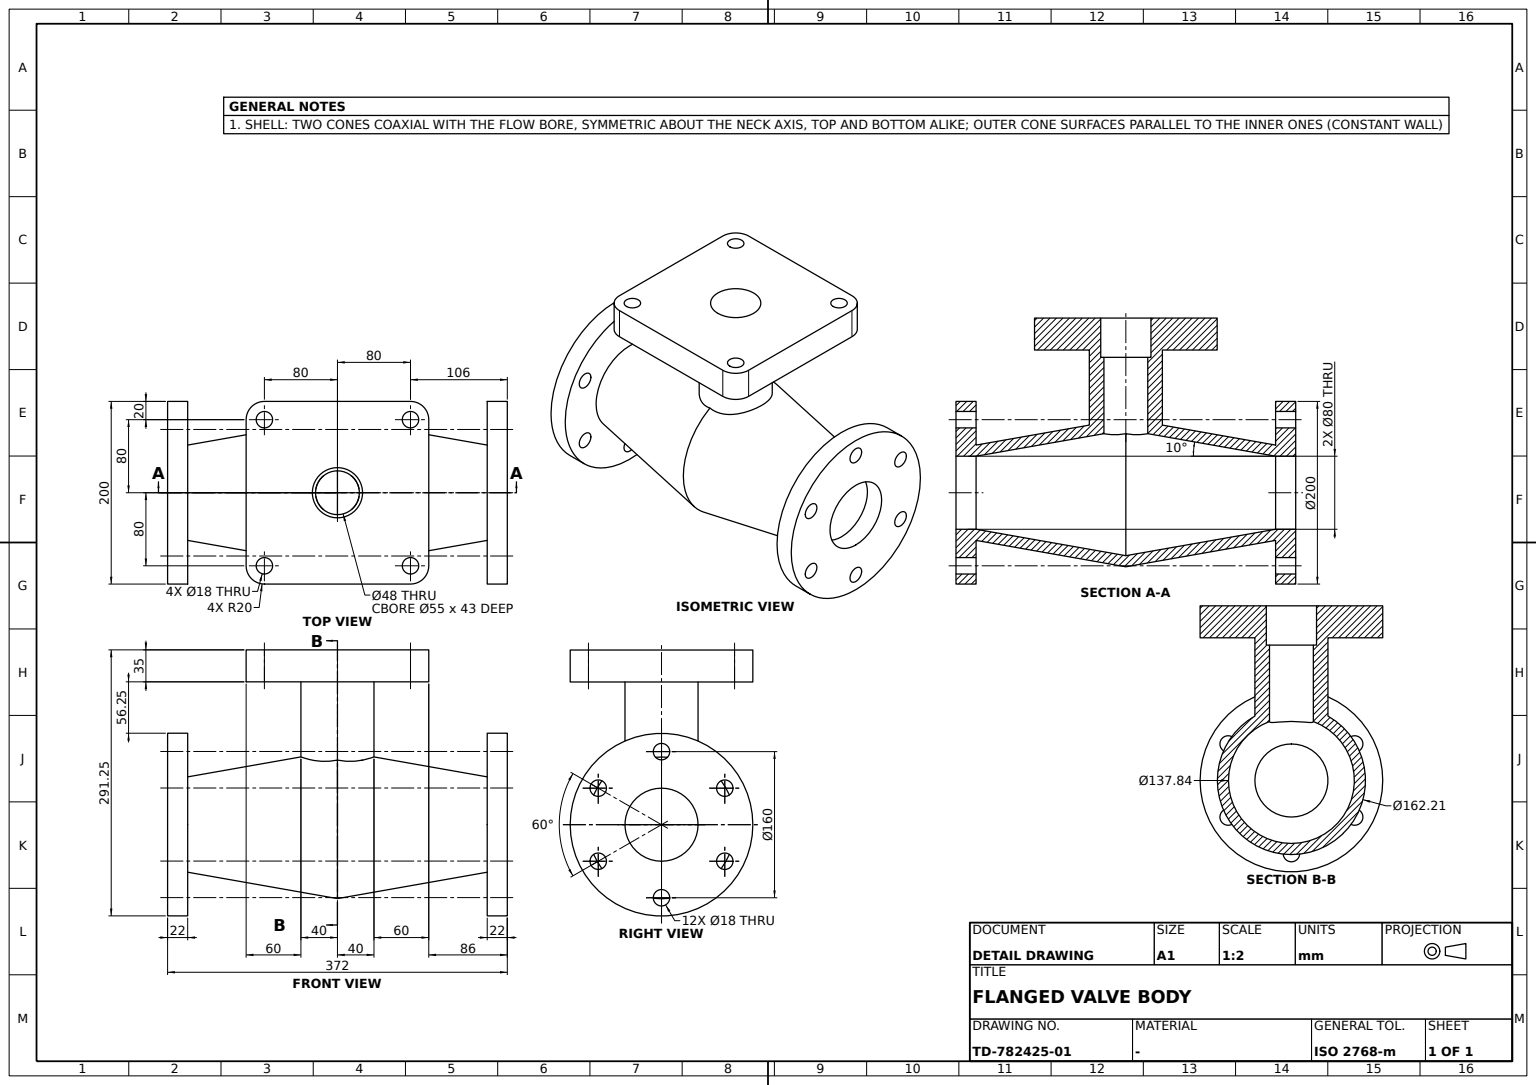
CATIA V5 part; units mm, degrees
sketch "Sketch1" plane through (0, 0, 0) normal (1, 0, 0) x (0, 1, 0)
  line L0 (0, 4.849) -> (164, -24.0686)
  point P0 (27.5, 0)
  point P1 (164, -24.0686)
  point P2 (-164, -24.0686)
  point P3 (-27.5, 0)
  line L1 (0, 4.849) -> (-164, -24.0686)
  point P4 (0, -9.4521)
  point P5 (-12, -9.4521)
  point P6 (12, -9.4521)
  line L2 (0, -7.3361) -> (-164, -36.2538)
  point P7 (-164, -36.2538)
  line L3 (-164, -24.0686) -> (-164, -36.2538)
  point P8 (164, -36.2538)
  point P9 (12, -9.4521)
  line L4 (0, -7.3361) -> (164, -36.2538)
  line L5 (164, -24.0686) -> (164, -36.2538)
  line L6 (-195.0876, -76.2538) -> (175.4473, -76.2538) construction
  point P10 (0, 4.849)
  dimension "angle L0 x axis" = 10
  dimension "distance P0 y axis" = 27.5
  dimension "distance P1 y axis" = 164
  dimension "distance L1 L2" = 12
  dimension "distance L6 P7" = 40
  dimension "distance P5 P6" = 24
  constraint coincidence P0 x-axis
  constraint coincidence P4 y-axis
  constraint coincidence P6 P9
  constraint coincidence P10 y-axis
  constraint coincidence P3 L1
  constraint coincidence P0 L0
  constraint coincidence P5 L2
  constraint coincidence P9 L4
  constraint symmetry P1 P2 y-axis
  constraint symmetry P0 P3 y-axis
  constraint symmetry L0 L1 y-axis
  constraint symmetry P7 P8 y-axis
  constraint symmetry P5 P9 y-axis
  constraint symmetry L2 L4 y-axis
  constraint vertical L3 y-axis
  constraint vertical L5 y-axis
  constraint horizontal L6 x-axis
revolve "Shaft1" add sketch "Sketch1" angle 360 about L6
sketch "Sketch3" plane through (0, 0, 0) normal (0, 0, 1) x (1, 0, 0)
  circle A0 centre (0, 0) radius 40
  dimension "radius A0" = 40
extrude "Pad1" add sketch "Sketch3" along normal blind 80 and the other way blind 10
sketch "Sketch4" plane through (0, 0, 80) normal (0, 0, 1) x (1, 0, 0)
  circle A0 centre (0, 0) radius 27.5
  dimension "radius A0" = 27.5
extrude "Pocket1" cut sketch "Sketch4" against normal blind 8
sketch "Sketch5" plane through (0, 0, 72) normal (0, 0, 1) x (1, 0, 0)
  circle A0 centre (0, 0) radius 24
  point P0 (24, 0)
  dimension "radius A0" = 24
  constraint coincidence A0 P0
  constraint coincidence P0 x-axis
extrude "Pocket2" cut sketch "Sketch5" against normal up to next
sketch "Sketch6" plane through (0, 0, 80) normal (0, 0, 1) x (1, 0, 0)
  circle A0 centre (0, 0) radius 27.5
  line L0 (100, 100) -> (100, -100)
  line L1 (100, -100) -> (-100, -100)
  line L2 (-100, -100) -> (-100, 100)
  line L3 (-100, 100) -> (100, 100)
  dimension "length L2" = 200
  dimension "length L3" = 200
  constraint vertical L0 y-axis
  constraint vertical L2 y-axis
  constraint horizontal L1 x-axis
  constraint horizontal L3 x-axis
  constraint equidistance L0 L2 origin
  constraint equidistance L1 L3 origin
extrude "Pad2" add sketch "Sketch6" along normal blind 35
fillet "Fillet1" radius 20 1 edges at (-100, 100, 97.5)
fillet "Fillet2" radius 20 1 edges at (-100, -100, 97.5)
fillet "Fillet3" radius 20 1 edges at (100, 100, 97.5)
fillet "Fillet4" radius 20 1 edges at (100, -100, 97.5)
sketch "Sketch7" plane through (0, 0, 115) normal (0, 0, 1) x (1, 0, 0)
  circle A0 centre (-80, 80) radius 9
  arc A1 (-80, 100) -> (-100, 80) centre (-80, 80) ccw construction
  circle A2 centre (80, 80) radius 9
  arc A3 (100, 80) -> (80, 100) centre (80, 80) ccw construction
  circle A4 centre (-80, -80) radius 9
  arc A5 (-100, -80) -> (-80, -100) centre (-80, -80) ccw construction
  circle A6 centre (80, -80) radius 9
  arc A7 (80, -100) -> (100, -80) centre (80, -80) ccw construction
  dimension "radius A0" = 9
  dimension "radius A2" = 9
  dimension "radius A4" = 9
  dimension "radius A6" = 9
  constraint concentricity A0 A1
  constraint concentricity A2 A3
  constraint concentricity A4 A5
  constraint concentricity A6 A7
extrude "Pocket3" cut sketch "Sketch7" against normal up to next
sketch "Sketch8" plane through (0, -164, 0) normal (0, -1, 0) x (1, 0, 0)
  circle A0 centre (0, -76.2538) radius 100
  point P0 (0, -76.2538)
  circle A1 centre (0, -76.2538) radius 52.1851 construction
  circle A2 centre (0, -76.2538) radius 40
  dimension "radius A0" = 100
  constraint coincidence P0 y-axis
  constraint concentricity A0 A1
extrude "Pad3" add sketch "Sketch8" along normal blind 22
sketch "Sketch9" plane through (0, 164, 0) normal (0, 1, 0) x (-1, 0, 0)
  circle A0 centre (0, -76.2538) radius 100
  point P0 (0, -76.2538)
  circle A1 centre (0, -76.2538) radius 100 construction
  circle A2 centre (0, -76.2538) radius 40
  constraint coincidence P0 y-axis
  constraint coincidence A0 A1
extrude "Pad4" add sketch "Sketch9" along normal blind 22
sketch "Sketch10" plane through (0, -186, 0) normal (0, -1, 0) x (1, 0, 0)
  circle A0 centre (0, -76.2538) radius 80 construction
  point P0 (0, -76.2538)
  circle A1 centre (0, -76.2538) radius 100 construction
  circle A2 centre (0, -156.2538) radius 9
  point P1 (0, -156.2538)
  circle A3 centre (0, 3.7462) radius 9
  point P2 (0, 3.7462)
  line L0 (0, -76.2538) -> (134.2866, 1.2767) construction
  point P3 (0, -76.2538)
  circle A4 centre (69.282, -36.2538) radius 9
  point P4 (69.282, -36.2538)
  line L1 (-187.4805, -76.2538) -> (187.4805, -76.2538) construction
  circle A5 centre (69.282, -116.2538) radius 9
  circle A6 centre (-69.282, -36.2538) radius 9
  circle A7 centre (-69.282, -116.2538) radius 9
  dimension "radius A0" = 80
  dimension "radius A2" = 9
  dimension "radius A3" = 9
  dimension "angle L0 y axis" = 60
  dimension "radius A4" = 9
  constraint coincidence P0 y-axis
  constraint coincidence P1 A0
  constraint coincidence P1 y-axis
  constraint coincidence P2 A0
  constraint coincidence P2 y-axis
  constraint coincidence P4 L0
  constraint coincidence P4 A0
  constraint coincidence P3 P0
  constraint concentricity A0 A1
  constraint midpoint L1 P0
  constraint horizontal L1 x-axis
  constraint symmetry A4 A5 L1
  constraint symmetry A4 A6 y-axis
  constraint symmetry A5 A7 y-axis
extrude "Pocket4" cut sketch "Sketch10" against normal up to next
sketch "Sketch11" plane through (0, 186, 0) normal (0, 1, 0) x (-1, 0, 0)
  circle A0 centre (0, -76.2538) radius 80 construction
  point P0 (0, -76.2538)
  circle A1 centre (0, -76.2538) radius 100 construction
  circle A2 centre (0, 3.7462) radius 9
  point P1 (0, 3.7462)
  circle A3 centre (0, -156.2538) radius 9
  point P2 (0, -156.2538)
  line L0 (-145.6152, -76.2538) -> (145.6152, -76.2538) construction
  line L1 (0, -76.2538) -> (119.6972, -7.1465) construction
  circle A4 centre (69.282, -36.2538) radius 9
  point P3 (69.282, -36.2538)
  circle A5 centre (-69.282, -36.2538) radius 9
  circle A6 centre (69.282, -116.2538) radius 9
  circle A7 centre (-69.282, -116.2538) radius 9
  dimension "radius A0" = 80
  dimension "radius A2" = 9
  dimension "radius A3" = 9
  dimension "angle L1 y axis" = 60
  dimension "radius A4" = 9
  constraint coincidence P0 y-axis
  constraint coincidence P1 A0
  constraint coincidence P1 y-axis
  constraint coincidence P2 A0
  constraint coincidence P2 y-axis
  constraint coincidence P3 L1
  constraint coincidence P3 A0
  constraint concentricity A0 A1
  constraint midpoint L0 P0
  constraint horizontal L0 x-axis
  constraint symmetry A4 A5 y-axis
  constraint symmetry A4 A6 L0
  constraint symmetry A5 A7 L0
extrude "Pocket5" cut sketch "Sketch11" against normal up to next
sketch "Sketch2" plane through (0, 0, 0) normal (0, 0, 1) x (1, 0, 0)
sketch "Sketch12" plane through (0, 0, 115) normal (0, 0, 1) x (1, 0, 0)
  circle A0 centre (0, 0) radius 80 construction
  dimension "radius A0" = 80
